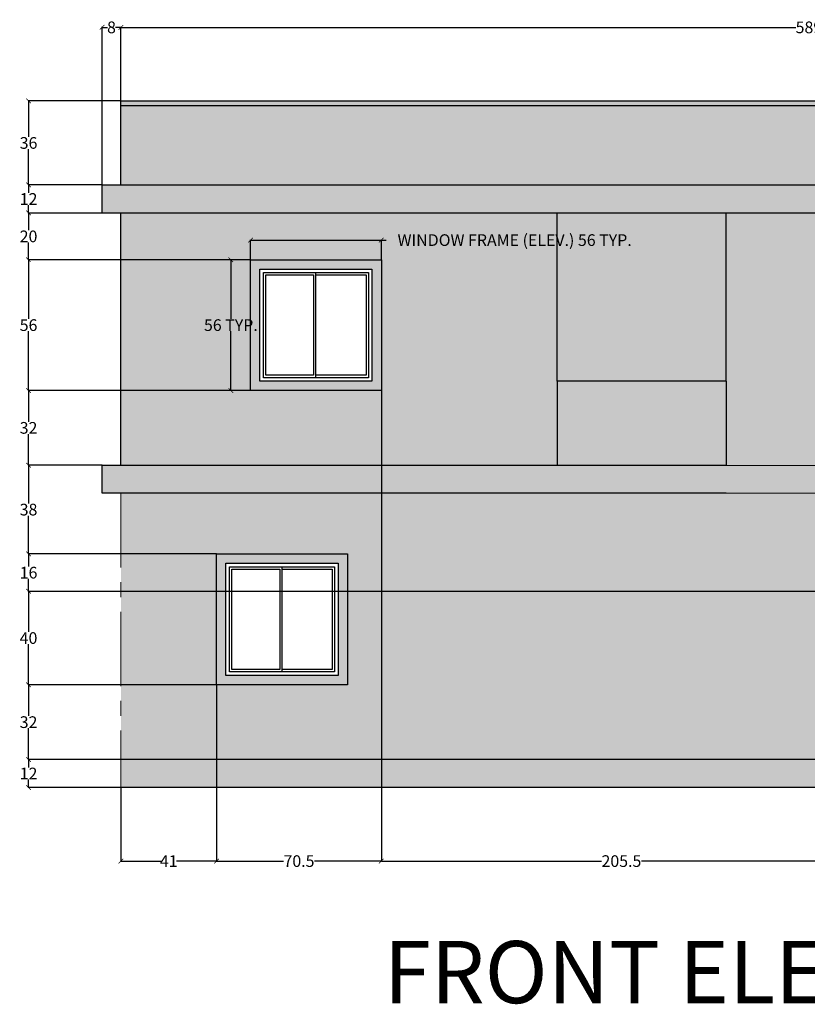
# Model space of a CAD drawing. Units: inches. Extents: x 1455 to 5994, y -182 to 2370.
# Tile 5 of 8: x 4241 to 4579, y -182 to 240. Entities that reach past the tile are written whole.
import ezdxf

# ---------------------------------------------------------------- set-up
doc = ezdxf.new("R2010")
doc.units = ezdxf.units.IN
doc.header["$MEASUREMENT"] = 0
doc.linetypes.add('CENTER', pattern=[50.8, 31.75, -6.35, 6.35, -6.35])
for name, color, linetype, lineweight in [('A-ANNO-DIMS', 2, 'Continuous', 18), ('A-ANNO-TEXT', 7, 'Continuous', 25), ('A-ELEV', 7, 'Continuous', 25), ('A-ELEV-PATT', 8, 'Continuous', 13), ('A-GRID', 8, 'CENTER', 18)]:
    doc.layers.add(name, color=color, linetype=linetype, lineweight=lineweight)
doc.styles.get("Standard").update_dxf_attribs({"font": 'arial.ttf'})
doc.dimstyles.get("Standard").update_dxf_attribs({"dimtxt": 5, "dimasz": 2, "dimexe": 0.18, "dimexo": 0.0625, "dimgap": 0.09, "dimtad": 0, "dimtih": 1, "dimtoh": 1, "dimdec": 1, "dimzin": 0, "dimdsep": 46, "dimlunit": 3, "dimtxsty": 'Standard', "dimblk": 'ARCHTICK', "dimcen": 0.09, "dimadec": 0, "dimazin": 0, "dimtfac": 1, "dimtdec": 1, "dimtofl": 0, "dimtmove": 0, "dimatfit": 3, "dimfxl": 1, "dimtolj": 1, "dimtzin": 0, "dimarcsym": 0})

# ---------------------------------------------------------------- blocks, each defined once
blk = doc.blocks.new('*U8')
for p, q in [((1.5, 1.5), (1.5, 46.5)), ((1.5, 46.5), (24, 46.5)), ((24, 1.5), (24, 46.5)), ((24, 46.5), (46.5, 46.5)), ((46.5, 46.5), (46.5, 1.5)), ((24, 1.5), (1.5, 1.5)), ((46.5, 1.5), (24, 1.5))]:
    blk.add_line(p, q)
blk.add_lwpolyline([(0, 0), (0, 48), (48, 48), (48, 0)], close=True)
for points in [[(23, 45.5), (23, 2.5), (2.5, 2.5), (2.5, 45.5), (23, 45.5)], [(24, 45.5), (45.5, 45.5), (45.5, 2.5), (24, 2.5)]]:
    blk.add_lwpolyline(points)
blk = doc.blocks.new('WIN-FRAME-ELEV')
for p, q in [((0, 0), (0, 56)), ((0, 56), (4, 56)), ((4, 56), (52, 56)), ((52, 56), (56, 56)), ((56, 56), (56, 4)), ((56, 4), (56, 0)), ((4, 0), (0, 0)), ((56, 0), (4, 0))]:
    blk.add_line(p, q)
blk = doc.blocks.new('_ArchTick')
at = {"color": 0, "linetype": 'ByBlock', "const_width": 0.15}
blk.add_lwpolyline([(-0.5, -0.5), (0.5, 0.5)], dxfattribs=at)
blk = doc.blocks.new('*D31')
at = {"layer": 'A-ANNO-DIMS', "color": 0, "lineweight": -2, "transparency": 16777216}
for p, q in [((4340.19, 137.16), (4340.19, 145.68)), ((4340.19, 145.5), (4396.19, 145.5)), ((4396.19, 137.16), (4396.19, 145.68)), ((4396.19, 145.5), (4398.19, 145.5))]:
    blk.add_line(p, q, dxfattribs=at)
at = {"layer": 'Defpoints', "color": 0, "lineweight": 25, "transparency": 16777216}
for p in [(4396.19, 145.5), (4340.19, 137.1), (4396.19, 137.1)]:
    blk.add_point(p, dxfattribs=at)
at = {"layer": 'A-ANNO-DIMS', "color": 0, "lineweight": -2, "transparency": 16777216, "xscale": 2, "yscale": 2, "zscale": 2, "rotation": 180}
blk.add_blockref('_ArchTick', (4340.19, 145.5), dxfattribs=at)
at = {"layer": 'A-ANNO-DIMS', "color": 0, "lineweight": -2, "transparency": 16777216, "xscale": 2, "yscale": 2, "zscale": 2}
blk.add_blockref('_ArchTick', (4396.19, 145.5), dxfattribs=at)
at = {"layer": 'A-ANNO-DIMS', "color": 0, "transparency": 16777216, "insert": (4453.24, 145.5), "char_height": 5, "attachment_point": 5}
blk.add_mtext('\\A1;WINDOW FRAME (ELEV.) 56 TYP.', dxfattribs=at)
blk = doc.blocks.new('*D32')
at = {"layer": 'A-ANNO-DIMS', "color": 0, "lineweight": -2, "transparency": 16777216}
for p, q in [((4340.13, 137.1), (4331.61, 137.1)), ((4331.79, 137.1), (4331.79, 111.74)), ((4331.79, 81.1), (4331.79, 106.45)), ((4340.13, 81.1), (4331.61, 81.1))]:
    blk.add_line(p, q, dxfattribs=at)
at = {"layer": 'Defpoints', "color": 0, "lineweight": 25, "transparency": 16777216}
for p in [(4331.79, 137.1), (4340.19, 137.1), (4340.19, 81.1)]:
    blk.add_point(p, dxfattribs=at)
at = {"layer": 'A-ANNO-DIMS', "color": 0, "lineweight": -2, "transparency": 16777216, "xscale": 2, "yscale": 2, "zscale": 2}
for p, rotation in [((4331.79, 137.1), 90), ((4331.79, 81.1), 270)]:
    blk.add_blockref('_ArchTick', p, dxfattribs=dict(at, rotation=rotation))
at = {"layer": 'A-ANNO-DIMS', "color": 0, "transparency": 16777216, "insert": (4331.79, 109.1), "char_height": 5, "attachment_point": 5}
blk.add_mtext('\\A1;56 TYP.', dxfattribs=at)
blk = doc.blocks.new('*D85')
at = {"layer": 'A-ANNO-DIMS', "color": 0, "lineweight": -2, "transparency": 16777216}
for p, q in [((4276.69, 169.16), (4276.69, 236.78)), ((4276.69, 236.6), (4278.95, 236.6)), ((4284.69, 236.6), (4282.43, 236.6)), ((4284.69, 205.16), (4284.69, 236.78))]:
    blk.add_line(p, q, dxfattribs=at)
at = {"layer": 'Defpoints', "color": 0, "lineweight": 25, "transparency": 16777216}
for p in [(4284.69, 236.6), (4284.69, 205.1), (4276.69, 169.1)]:
    blk.add_point(p, dxfattribs=at)
at = {"layer": 'A-ANNO-DIMS', "color": 0, "lineweight": -2, "transparency": 16777216, "xscale": 2, "yscale": 2, "zscale": 2, "rotation": 180}
blk.add_blockref('_ArchTick', (4276.69, 236.6), dxfattribs=at)
at = {"layer": 'A-ANNO-DIMS', "color": 0, "lineweight": -2, "transparency": 16777216, "xscale": 2, "yscale": 2, "zscale": 2}
blk.add_blockref('_ArchTick', (4284.69, 236.6), dxfattribs=at)
at = {"layer": 'A-ANNO-DIMS', "color": 0, "transparency": 16777216, "insert": (4280.69, 236.6), "char_height": 5, "attachment_point": 5}
blk.add_mtext('\\A1;8', dxfattribs=at)
blk = doc.blocks.new('*D86')
at = {"layer": 'A-ANNO-DIMS', "color": 0, "lineweight": -2, "transparency": 16777216}
for p, q in [((4284.69, 205.16), (4284.69, 236.78)), ((4284.69, 236.6), (4573.57, 236.6)), ((4873.69, 236.6), (4584.81, 236.6)), ((4873.69, 205.16), (4873.69, 236.78))]:
    blk.add_line(p, q, dxfattribs=at)
at = {"layer": 'Defpoints', "color": 0, "lineweight": 25, "transparency": 16777216}
for p in [(4873.69, 236.6), (4284.69, 205.1), (4873.69, 205.1)]:
    blk.add_point(p, dxfattribs=at)
at = {"layer": 'A-ANNO-DIMS', "color": 0, "lineweight": -2, "transparency": 16777216, "xscale": 2, "yscale": 2, "zscale": 2, "rotation": 180}
blk.add_blockref('_ArchTick', (4284.69, 236.6), dxfattribs=at)
at = {"layer": 'A-ANNO-DIMS', "color": 0, "lineweight": -2, "transparency": 16777216, "xscale": 2, "yscale": 2, "zscale": 2}
blk.add_blockref('_ArchTick', (4873.69, 236.6), dxfattribs=at)
at = {"layer": 'A-ANNO-DIMS', "color": 0, "transparency": 16777216, "insert": (4579.19, 236.6), "char_height": 5, "attachment_point": 5}
blk.add_mtext('\\A1;589', dxfattribs=at)
blk = doc.blocks.new('*D87')
at = {"layer": 'A-ANNO-DIMS', "color": 0, "lineweight": -2, "transparency": 16777216}
for p, q in [((4325.69, -44.97), (4325.69, -120.58)), ((4284.69, -88.97), (4284.69, -120.58)), ((4284.69, -120.4), (4301.9, -120.4)), ((4325.69, -120.4), (4308.48, -120.4))]:
    blk.add_line(p, q, dxfattribs=at)
at = {"layer": 'Defpoints', "color": 0, "lineweight": 25, "transparency": 16777216}
for p in [(4325.69, -44.9), (4284.69, -88.9), (4325.69, -120.4)]:
    blk.add_point(p, dxfattribs=at)
at = {"layer": 'A-ANNO-DIMS', "color": 0, "lineweight": -2, "transparency": 16777216, "xscale": 2, "yscale": 2, "zscale": 2, "rotation": 180}
blk.add_blockref('_ArchTick', (4284.69, -120.4), dxfattribs=at)
at = {"layer": 'A-ANNO-DIMS', "color": 0, "lineweight": -2, "transparency": 16777216, "xscale": 2, "yscale": 2, "zscale": 2}
blk.add_blockref('_ArchTick', (4325.69, -120.4), dxfattribs=at)
at = {"layer": 'A-ANNO-DIMS', "color": 0, "transparency": 16777216, "insert": (4305.19, -120.4), "char_height": 5, "attachment_point": 5}
blk.add_mtext('\\A1;41', dxfattribs=at)
blk = doc.blocks.new('*D88')
at = {"layer": 'A-ANNO-DIMS', "color": 0, "lineweight": -2, "transparency": 16777216}
for p, q in [((4396.19, 81.03), (4396.19, -120.58)), ((4325.69, -44.97), (4325.69, -120.58)), ((4325.69, -120.4), (4354.36, -120.4)), ((4396.19, -120.4), (4367.52, -120.4))]:
    blk.add_line(p, q, dxfattribs=at)
at = {"layer": 'Defpoints', "color": 0, "lineweight": 25, "transparency": 16777216}
for p in [(4396.19, 81.1), (4325.69, -44.9), (4396.19, -120.4)]:
    blk.add_point(p, dxfattribs=at)
at = {"layer": 'A-ANNO-DIMS', "color": 0, "lineweight": -2, "transparency": 16777216, "xscale": 2, "yscale": 2, "zscale": 2, "rotation": 180}
blk.add_blockref('_ArchTick', (4325.69, -120.4), dxfattribs=at)
at = {"layer": 'A-ANNO-DIMS', "color": 0, "lineweight": -2, "transparency": 16777216, "xscale": 2, "yscale": 2, "zscale": 2}
blk.add_blockref('_ArchTick', (4396.19, -120.4), dxfattribs=at)
at = {"layer": 'A-ANNO-DIMS', "color": 0, "transparency": 16777216, "insert": (4360.94, -120.4), "char_height": 5, "attachment_point": 5}
blk.add_mtext('\\A1;70.5', dxfattribs=at)
blk = doc.blocks.new('*D89')
at = {"layer": 'A-ANNO-DIMS', "color": 0, "lineweight": -2, "transparency": 16777216}
for p, q in [((4396.19, 81.03), (4396.19, -120.58)), ((4601.69, 81.03), (4601.69, -120.58)), ((4396.19, -120.4), (4490.35, -120.4)), ((4601.69, -120.4), (4507.53, -120.4))]:
    blk.add_line(p, q, dxfattribs=at)
at = {"layer": 'Defpoints', "color": 0, "lineweight": 25, "transparency": 16777216}
for p in [(4396.19, 81.1), (4601.69, 81.1), (4601.69, -120.4)]:
    blk.add_point(p, dxfattribs=at)
at = {"layer": 'A-ANNO-DIMS', "color": 0, "lineweight": -2, "transparency": 16777216, "xscale": 2, "yscale": 2, "zscale": 2, "rotation": 180}
blk.add_blockref('_ArchTick', (4396.19, -120.4), dxfattribs=at)
at = {"layer": 'A-ANNO-DIMS', "color": 0, "lineweight": -2, "transparency": 16777216, "xscale": 2, "yscale": 2, "zscale": 2}
blk.add_blockref('_ArchTick', (4601.69, -120.4), dxfattribs=at)
at = {"layer": 'A-ANNO-DIMS', "color": 0, "transparency": 16777216, "insert": (4498.94, -120.4), "char_height": 5, "attachment_point": 5}
blk.add_mtext('\\A1;205.5', dxfattribs=at)
blk = doc.blocks.new('*D96')
at = {"layer": 'A-ANNO-DIMS', "color": 0, "lineweight": -2, "transparency": 16777216}
for p, q in [((4284.63, -76.9), (4245.01, -76.9)), ((4245.19, -76.9), (4245.19, -80.3)), ((4245.19, -88.9), (4245.19, -85.5)), ((4284.63, -88.9), (4245.01, -88.9))]:
    blk.add_line(p, q, dxfattribs=at)
at = {"layer": 'Defpoints', "color": 0, "lineweight": 25, "transparency": 16777216}
for p in [(4245.19, -76.9), (4284.69, -76.9), (4284.69, -88.9)]:
    blk.add_point(p, dxfattribs=at)
at = {"layer": 'A-ANNO-DIMS', "color": 0, "lineweight": -2, "transparency": 16777216, "xscale": 2, "yscale": 2, "zscale": 2}
for p, rotation in [((4245.19, -76.9), 90), ((4245.19, -88.9), 270)]:
    blk.add_blockref('_ArchTick', p, dxfattribs=dict(at, rotation=rotation))
at = {"layer": 'A-ANNO-DIMS', "color": 0, "transparency": 16777216, "insert": (4245.19, -82.9), "char_height": 5, "attachment_point": 5}
blk.add_mtext('\\A1;12', dxfattribs=at)
blk = doc.blocks.new('*D97')
at = {"layer": 'A-ANNO-DIMS', "color": 0, "lineweight": -2, "transparency": 16777216}
for p, q in [((4325.63, -44.9), (4245.01, -44.9)), ((4245.19, -44.9), (4245.19, -58.26)), ((4245.19, -76.9), (4245.19, -63.55)), ((4284.63, -76.9), (4245.01, -76.9))]:
    blk.add_line(p, q, dxfattribs=at)
at = {"layer": 'Defpoints', "color": 0, "lineweight": 25, "transparency": 16777216}
for p in [(4245.19, -44.9), (4325.69, -44.9), (4284.69, -76.9)]:
    blk.add_point(p, dxfattribs=at)
at = {"layer": 'A-ANNO-DIMS', "color": 0, "lineweight": -2, "transparency": 16777216, "xscale": 2, "yscale": 2, "zscale": 2}
for p, rotation in [((4245.19, -44.9), 90), ((4245.19, -76.9), 270)]:
    blk.add_blockref('_ArchTick', p, dxfattribs=dict(at, rotation=rotation))
at = {"layer": 'A-ANNO-DIMS', "color": 0, "transparency": 16777216, "insert": (4245.19, -60.9), "char_height": 5, "attachment_point": 5}
blk.add_mtext('\\A1;32', dxfattribs=at)
blk = doc.blocks.new('*D98')
at = {"layer": 'A-ANNO-DIMS', "color": 0, "lineweight": -2, "transparency": 16777216}
for p, q in [((4619.63, -4.9), (4245.01, -4.9)), ((4245.19, -4.9), (4245.19, -22.26)), ((4245.19, -44.9), (4245.19, -27.55)), ((4325.63, -44.9), (4245.01, -44.9))]:
    blk.add_line(p, q, dxfattribs=at)
at = {"layer": 'Defpoints', "color": 0, "lineweight": 25, "transparency": 16777216}
for p in [(4245.19, -4.9), (4619.69, -4.9), (4325.69, -44.9)]:
    blk.add_point(p, dxfattribs=at)
at = {"layer": 'A-ANNO-DIMS', "color": 0, "lineweight": -2, "transparency": 16777216, "xscale": 2, "yscale": 2, "zscale": 2}
for p, rotation in [((4245.19, -4.9), 90), ((4245.19, -44.9), 270)]:
    blk.add_blockref('_ArchTick', p, dxfattribs=dict(at, rotation=rotation))
at = {"layer": 'A-ANNO-DIMS', "color": 0, "transparency": 16777216, "insert": (4245.19, -24.9), "char_height": 5, "attachment_point": 5}
blk.add_mtext('\\A1;40', dxfattribs=at)
blk = doc.blocks.new('*D99')
at = {"layer": 'A-ANNO-DIMS', "color": 0, "lineweight": -2, "transparency": 16777216}
for p, q in [((4325.63, 11.1), (4245.01, 11.1)), ((4245.19, 11.1), (4245.19, 5.74)), ((4245.19, -4.9), (4245.19, 0.45)), ((4619.63, -4.9), (4245.01, -4.9))]:
    blk.add_line(p, q, dxfattribs=at)
at = {"layer": 'Defpoints', "color": 0, "lineweight": 25, "transparency": 16777216}
for p in [(4245.19, 11.1), (4325.69, 11.1), (4619.69, -4.9)]:
    blk.add_point(p, dxfattribs=at)
at = {"layer": 'A-ANNO-DIMS', "color": 0, "lineweight": -2, "transparency": 16777216, "xscale": 2, "yscale": 2, "zscale": 2}
for p, rotation in [((4245.19, 11.1), 90), ((4245.19, -4.9), 270)]:
    blk.add_blockref('_ArchTick', p, dxfattribs=dict(at, rotation=rotation))
at = {"layer": 'A-ANNO-DIMS', "color": 0, "transparency": 16777216, "insert": (4245.19, 3.1), "char_height": 5, "attachment_point": 5}
blk.add_mtext('\\A1;16', dxfattribs=at)
blk = doc.blocks.new('*D100')
at = {"layer": 'A-ANNO-DIMS', "color": 0, "lineweight": -2, "transparency": 16777216}
for p, q in [((4276.63, 49.1), (4245.01, 49.1)), ((4245.19, 49.1), (4245.19, 32.74)), ((4245.19, 11.1), (4245.19, 27.45)), ((4325.63, 11.1), (4245.01, 11.1))]:
    blk.add_line(p, q, dxfattribs=at)
at = {"layer": 'Defpoints', "color": 0, "lineweight": 25, "transparency": 16777216}
for p in [(4245.19, 49.1), (4276.69, 49.1), (4325.69, 11.1)]:
    blk.add_point(p, dxfattribs=at)
at = {"layer": 'A-ANNO-DIMS', "color": 0, "lineweight": -2, "transparency": 16777216, "xscale": 2, "yscale": 2, "zscale": 2}
for p, rotation in [((4245.19, 49.1), 90), ((4245.19, 11.1), 270)]:
    blk.add_blockref('_ArchTick', p, dxfattribs=dict(at, rotation=rotation))
at = {"layer": 'A-ANNO-DIMS', "color": 0, "transparency": 16777216, "insert": (4245.19, 30.1), "char_height": 5, "attachment_point": 5}
blk.add_mtext('\\A1;38', dxfattribs=at)
blk = doc.blocks.new('*D101')
at = {"layer": 'A-ANNO-DIMS', "color": 0, "lineweight": -2, "transparency": 16777216}
for p, q in [((4340.13, 81.1), (4245.01, 81.1)), ((4245.19, 81.1), (4245.19, 67.74)), ((4245.19, 49.1), (4245.19, 62.45)), ((4276.63, 49.1), (4245.01, 49.1))]:
    blk.add_line(p, q, dxfattribs=at)
at = {"layer": 'Defpoints', "color": 0, "lineweight": 25, "transparency": 16777216}
for p in [(4245.19, 81.1), (4340.19, 81.1), (4276.69, 49.1)]:
    blk.add_point(p, dxfattribs=at)
at = {"layer": 'A-ANNO-DIMS', "color": 0, "lineweight": -2, "transparency": 16777216, "xscale": 2, "yscale": 2, "zscale": 2}
for p, rotation in [((4245.19, 81.1), 90), ((4245.19, 49.1), 270)]:
    blk.add_blockref('_ArchTick', p, dxfattribs=dict(at, rotation=rotation))
at = {"layer": 'A-ANNO-DIMS', "color": 0, "transparency": 16777216, "insert": (4245.19, 65.1), "char_height": 5, "attachment_point": 5}
blk.add_mtext('\\A1;32', dxfattribs=at)
blk = doc.blocks.new('*D102')
at = {"layer": 'A-ANNO-DIMS', "color": 0, "lineweight": -2, "transparency": 16777216}
for p, q in [((4340.13, 137.1), (4245.01, 137.1)), ((4245.19, 137.1), (4245.19, 111.74)), ((4245.19, 81.1), (4245.19, 106.45)), ((4340.13, 81.1), (4245.01, 81.1))]:
    blk.add_line(p, q, dxfattribs=at)
at = {"layer": 'Defpoints', "color": 0, "lineweight": 25, "transparency": 16777216}
for p in [(4245.19, 137.1), (4340.19, 137.1), (4340.19, 81.1)]:
    blk.add_point(p, dxfattribs=at)
at = {"layer": 'A-ANNO-DIMS', "color": 0, "lineweight": -2, "transparency": 16777216, "xscale": 2, "yscale": 2, "zscale": 2}
for p, rotation in [((4245.19, 137.1), 90), ((4245.19, 81.1), 270)]:
    blk.add_blockref('_ArchTick', p, dxfattribs=dict(at, rotation=rotation))
at = {"layer": 'A-ANNO-DIMS', "color": 0, "transparency": 16777216, "insert": (4245.19, 109.1), "char_height": 5, "attachment_point": 5}
blk.add_mtext('\\A1;56', dxfattribs=at)
blk = doc.blocks.new('*D103')
at = {"layer": 'A-ANNO-DIMS', "color": 0, "lineweight": -2, "transparency": 16777216}
for p, q in [((4276.63, 157.1), (4245.01, 157.1)), ((4245.19, 157.1), (4245.19, 149.74)), ((4245.19, 137.1), (4245.19, 144.45)), ((4340.13, 137.1), (4245.01, 137.1))]:
    blk.add_line(p, q, dxfattribs=at)
at = {"layer": 'Defpoints', "color": 0, "lineweight": 25, "transparency": 16777216}
for p in [(4245.19, 157.1), (4276.69, 157.1), (4340.19, 137.1)]:
    blk.add_point(p, dxfattribs=at)
at = {"layer": 'A-ANNO-DIMS', "color": 0, "lineweight": -2, "transparency": 16777216, "xscale": 2, "yscale": 2, "zscale": 2}
for p, rotation in [((4245.19, 157.1), 90), ((4245.19, 137.1), 270)]:
    blk.add_blockref('_ArchTick', p, dxfattribs=dict(at, rotation=rotation))
at = {"layer": 'A-ANNO-DIMS', "color": 0, "transparency": 16777216, "insert": (4245.19, 147.1), "char_height": 5, "attachment_point": 5}
blk.add_mtext('\\A1;20', dxfattribs=at)
blk = doc.blocks.new('*D104')
at = {"layer": 'A-ANNO-DIMS', "color": 0, "lineweight": -2, "transparency": 16777216}
for p, q in [((4276.63, 169.1), (4245.01, 169.1)), ((4245.19, 169.1), (4245.19, 165.7)), ((4245.19, 157.1), (4245.19, 160.5)), ((4276.63, 157.1), (4245.01, 157.1))]:
    blk.add_line(p, q, dxfattribs=at)
at = {"layer": 'Defpoints', "color": 0, "lineweight": 25, "transparency": 16777216}
for p in [(4245.19, 169.1), (4276.69, 169.1), (4276.69, 157.1)]:
    blk.add_point(p, dxfattribs=at)
at = {"layer": 'A-ANNO-DIMS', "color": 0, "lineweight": -2, "transparency": 16777216, "xscale": 2, "yscale": 2, "zscale": 2}
for p, rotation in [((4245.19, 169.1), 90), ((4245.19, 157.1), 270)]:
    blk.add_blockref('_ArchTick', p, dxfattribs=dict(at, rotation=rotation))
at = {"layer": 'A-ANNO-DIMS', "color": 0, "transparency": 16777216, "insert": (4245.19, 163.1), "char_height": 5, "attachment_point": 5}
blk.add_mtext('\\A1;12', dxfattribs=at)
blk = doc.blocks.new('*D105')
at = {"layer": 'A-ANNO-DIMS', "color": 0, "lineweight": -2, "transparency": 16777216}
for p, q in [((4284.63, 205.1), (4245.01, 205.1)), ((4245.19, 205.1), (4245.19, 189.74)), ((4245.19, 169.1), (4245.19, 184.45)), ((4276.63, 169.1), (4245.01, 169.1))]:
    blk.add_line(p, q, dxfattribs=at)
at = {"layer": 'Defpoints', "color": 0, "lineweight": 25, "transparency": 16777216}
for p in [(4245.19, 205.1), (4284.69, 205.1), (4276.69, 169.1)]:
    blk.add_point(p, dxfattribs=at)
at = {"layer": 'A-ANNO-DIMS', "color": 0, "lineweight": -2, "transparency": 16777216, "xscale": 2, "yscale": 2, "zscale": 2}
for p, rotation in [((4245.19, 205.1), 90), ((4245.19, 169.1), 270)]:
    blk.add_blockref('_ArchTick', p, dxfattribs=dict(at, rotation=rotation))
at = {"layer": 'A-ANNO-DIMS', "color": 0, "transparency": 16777216, "insert": (4245.19, 187.1), "char_height": 5, "attachment_point": 5}
blk.add_mtext('\\A1;36', dxfattribs=at)

msp = doc.modelspace()

# ---------------------------------------------------------------- hatches: boundary and pattern name
at = {"layer": 'A-ELEV-PATT', "transparency": 33554641}
h = msp.add_hatch(color=256, dxfattribs=at)
h.dxf.hatch_style = 1
h.paths.add_polyline_path([(4873.6884, 205.0969), (4284.6884, 205.0969), (4284.6884, 203.0969), (4873.6884, 203.0969)])
h = msp.add_hatch(color=256, dxfattribs=at)
h.dxf.hatch_style = 1
h.paths.add_polyline_path([(4873.6884, 203.0969), (4284.6884, 203.0969), (4284.6884, 169.0969), (4768.6884, 169.0969), (4864.6884, 169.0969), (4873.6884, 169.0969)])
h = msp.add_hatch(color=256, dxfattribs=at)
h.dxf.hatch_style = 1
h.paths.add_polyline_path([(4768.6884, 169.0969), (4284.6884, 169.0969), (4276.6884, 169.0969), (4276.6884, 157.0969), (4756.6884, 157.0969), (4756.6884, 49.0187), (4719.7422, 49.0288), (4719.7422, 49.0261), (4713.167, 49.0261), (4704.4367, 49.0287), (4704.4367, 49.0261), (4697.8615, 49.0261), (4689.1312, 49.0288), (4689.1312, 49.0261), (4682.556, 49.0261), (4673.8258, 49.029), (4673.8258, 49.0261), (4667.2505, 49.0261), (4471.4513, 49.0969), (4284.6884, 49.0969), (4276.6884, 49.0969), (4276.6884, 37.0915), (4543.7991, 37.0915), (4768.6843, 37.0146)])
h = msp.add_hatch(color=256, dxfattribs=at)
h.dxf.hatch_style = 1
h.paths.add_polyline_path([(4873.6884, 169.0969), (4864.6884, 169.0969), (4864.6884, 85.0969), (4864.6884, 49.0146), (4864.6884, 43.0969), (4864.6884, -70.9031), (4864.6884, -76.9031), (4861.6884, -76.9031), (4837.6884, -76.9031), (4834.6884, -76.9031), (4768.6884, -76.9031), (4763.6884, -76.9031), (4284.6884, -76.9031), (4284.6884, -88.9031), (4873.6884, -88.9031)])
h = msp.add_hatch(color=256, dxfattribs=at)
h.dxf.hatch_style = 1
h.paths.add_polyline_path([(4471.4513, 157.0969), (4284.6884, 157.0969), (4284.6884, 49.0969), (4471.4513, 49.0969), (4471.4513, 85.0969)])
h.paths.add_polyline_path([(4396.1884, 85.0969), (4396.1884, 81.0969), (4344.1884, 81.0969), (4340.1884, 81.0969), (4340.1884, 137.0969), (4344.1884, 137.0969), (4392.1884, 137.0969), (4396.1884, 137.0969)], flags=16)
h.paths.add_polyline_path([(4607.6884, 37.0697), (4543.7991, 37.0915), (4284.6884, 37.0915), (4284.6884, -76.9031), (4607.6884, -76.9031)])
h.paths.add_polyline_path([(4381.6884, -40.9031), (4381.6884, -44.9031), (4329.6884, -44.9031), (4325.6884, -44.9031), (4325.6884, 11.0969), (4329.6884, 11.0969), (4377.6884, 11.0969), (4381.6884, 11.0969)], flags=16)
h.paths.add_polyline_path([(4377.6884, -40.9031), (4329.6884, -40.9031), (4329.6884, 7.0969), (4377.6884, 7.0969)], flags=0)
h.paths.add_polyline_path([(4376.1884, -39.4031), (4353.6884, -39.4031), (4331.1884, -39.4031), (4331.1884, 5.5969), (4353.6884, 5.5969), (4376.1884, 5.5969)], flags=0)
h.paths.add_polyline_path([(4375.1884, -38.4031), (4353.6884, -38.4031), (4353.6884, 4.5969), (4375.1884, 4.5969)], flags=0)
h.paths.add_polyline_path([(4352.6884, -38.4031), (4332.1884, -38.4031), (4332.1884, 4.5969), (4352.6884, 4.5969)], flags=0)
h.paths.add_polyline_path([(4667.2505, 157.0969), (4543.8032, 157.0969), (4543.8032, 85.0969), (4543.8032, 49.0771), (4667.2505, 49.0432)])
h.paths.add_polyline_path([(4601.6884, 81.0969), (4601.6884, 137.0969), (4605.6884, 137.0969), (4653.6884, 137.0969), (4657.6884, 137.0969), (4657.6884, 81.0969)], flags=16)
h.paths.add_polyline_path([(4543.8032, 157.0969), (4471.4513, 157.0969), (4471.4513, 85.0969), (4543.8032, 85.0969)])
h.paths.add_polyline_path([(4763.6884, 37.0163), (4619.6884, 37.0656), (4619.6884, -4.9031), (4643.6884, -4.9031), (4667.6884, -4.9031), (4667.6884, -76.9031), (4763.6884, -76.9031)])
h.paths.add_polyline_path([(4864.6884, 43.0969), (4768.6884, 43.0969), (4768.6884, -76.9031), (4834.6884, -76.9031), (4834.6884, -4.9031), (4864.6884, -4.9031)])
h = msp.add_hatch(color=256, dxfattribs=at)
h.dxf.hatch_style = 1
h.paths.add_polyline_path([(4396.1884, 137.0969), (4392.1884, 137.0969), (4344.1884, 137.0969), (4340.1884, 137.0969), (4340.1884, 81.0969), (4344.1884, 81.0969), (4396.1884, 81.0969), (4396.1884, 85.0969)])
h.paths.add_polyline_path([(4344.1884, 133.0969), (4392.1884, 133.0969), (4392.1884, 85.0969), (4344.1884, 85.0969)], flags=16)
h.paths.add_polyline_path([(4345.6884, 131.5969), (4368.1884, 131.5969), (4390.6884, 131.5969), (4390.6884, 86.5969), (4368.1884, 86.5969), (4345.6884, 86.5969)], flags=0)
h.paths.add_polyline_path([(4346.6884, 130.5969), (4367.1884, 130.5969), (4367.1884, 87.5969), (4346.6884, 87.5969)], flags=0)
h.paths.add_polyline_path([(4368.1884, 130.5969), (4389.6884, 130.5969), (4389.6884, 87.5969), (4368.1884, 87.5969)], flags=0)
h.paths.add_polyline_path([(4657.6884, 137.0969), (4653.6884, 137.0969), (4605.6884, 137.0969), (4601.6884, 137.0969), (4601.6884, 81.0969), (4657.6884, 81.0969)])
h.paths.add_polyline_path([(4653.6884, 133.0969), (4653.6884, 85.0969), (4605.6884, 85.0969), (4605.6884, 133.0969)], flags=16)
h.paths.add_polyline_path([(4629.6884, 131.5969), (4652.1884, 131.5969), (4652.1884, 86.5969), (4629.6884, 86.5969), (4607.1884, 86.5969), (4607.1884, 131.5969)], flags=0)
h.paths.add_polyline_path([(4628.6884, 130.5969), (4628.6884, 87.5969), (4608.1884, 87.5969), (4608.1884, 130.5969)], flags=0)
h.paths.add_polyline_path([(4629.6884, 130.5969), (4651.1884, 130.5969), (4651.1884, 87.5969), (4629.6884, 87.5969)], flags=0)
h.paths.add_polyline_path([(4381.6884, 11.0969), (4377.6884, 11.0969), (4329.6884, 11.0969), (4325.6884, 11.0969), (4325.6884, -44.9031), (4329.6884, -44.9031), (4381.6884, -44.9031), (4381.6884, -40.9031)])
h.paths.add_polyline_path([(4377.6884, 7.0969), (4377.6884, -40.9031), (4329.6884, -40.9031), (4329.6884, 7.0969)], flags=16)
h.paths.add_polyline_path([(4353.6884, 5.5969), (4376.1884, 5.5969), (4376.1884, -39.4031), (4353.6884, -39.4031), (4331.1884, -39.4031), (4331.1884, 5.5969)], flags=0)
h.paths.add_polyline_path([(4353.6884, 4.5969), (4375.1884, 4.5969), (4375.1884, -38.4031), (4353.6884, -38.4031)], flags=0)
h.paths.add_polyline_path([(4352.6884, -38.4031), (4332.1884, -38.4031), (4332.1884, 4.5969), (4352.6884, 4.5969)], flags=0)
at = {"layer": 'A-ELEV-PATT', "transparency": 33554666}
h = msp.add_hatch(color=256, dxfattribs=at)
h.dxf.hatch_style = 1
h.paths.add_polyline_path([(4864.6884, 85.0969), (4768.6884, 85.0969), (4768.6884, 49.0969), (4864.6884, 49.0969)])
h.paths.add_polyline_path([(4543.8032, 85.0969), (4471.4513, 85.0969), (4471.4513, 49.0969), (4543.8032, 49.0969)])

# ---------------------------------------------------------------- linework, layer by layer
at = {"layer": 'A-ELEV'}
for p, q in [((4284.6884, 169.0969), (4284.6884, 205.0969)), ((4284.6884, 205.0969), (4873.6884, 205.0969)), ((4284.6884, 203.0969), (4873.6884, 203.0969)), ((4284.6884, 49.0969), (4284.6884, 157.0969)), ((4471.4513, 85.0969), (4471.4513, 157.0969)), ((4543.8032, 85.0969), (4543.8032, 157.0969)), ((4471.4513, 85.0969), (4471.4513, 49.0969)), ((4543.8032, 85.0969), (4471.4513, 85.0969)), ((4543.8032, 85.0969), (4543.8032, 49.0915)), ((4471.4513, 49.0969), (4543.8032, 49.0969)), ((4763.6884, -76.9031), (4284.6884, -76.9031)), ((4873.6884, -88.9031), (4284.6884, -88.9031))]:
    msp.add_line(p, q, dxfattribs=at)
msp.add_lwpolyline([(4756.6884, 49.0146), (4756.6884, 157.0969), (4276.6884, 157.0969), (4276.6884, 169.0969), (4284.6884, 169.0969), (4768.6884, 169.0969), (4768.6843, 37.0146), (4543.7991, 37.0915), (4276.6884, 37.0915), (4276.6884, 49.0969), (4284.6884, 49.0969), (4471.4513, 49.0969), (4756.6884, 49.0187)], dxfattribs=at)
at = {"layer": 'A-GRID'}
msp.add_line((4284.6884, 37.0915), (4284.6884, -88.9031), dxfattribs=at)

# ---------------------------------------------------------------- block references
at = {"layer": 'A-ELEV'}
for name, p in [('WIN-FRAME-ELEV', (4340.188, 81.097)), ('*U8', (4344.1884, 85.0969)), ('WIN-FRAME-ELEV', (4325.688, -44.903)), ('*U8', (4329.6884, -40.9031))]:
    msp.add_blockref(name, p, dxfattribs=at)

# ---------------------------------------------------------------- texts
at = {"layer": 'A-ANNO-TEXT'}
msp.add_text('FRONT ELEVATION', height=26.640459, dxfattribs=at).set_placement((4397.2929, -181.252))

# ---------------------------------------------------------------- dimensions: what is measured, and where the dimension line sits
at = {"layer": 'A-ANNO-DIMS'}
for base, p1, p2, override, picture, middle in [((4284.6884, 236.5969), (4276.6884, 169.0969), (4284.6884, 205.0969), {"dimdec": 0, "dimlfac": 1, "dimrnd": 0, "dimzin": 0, "dimdsep": 46, "dimlunit": 2}, '*D85', (4280.6884, 236.5969)), ((4873.6884, 236.5969), (4284.6884, 205.0969), (4873.6884, 205.0969), {"dimdec": 0, "dimlfac": 1, "dimrnd": 0, "dimzin": 0, "dimdsep": 46, "dimlunit": 2}, '*D86', (4579.1884, 236.5969)), ((4396.1884, -120.4031), (4325.6884, -44.9031), (4396.1884, 81.0969), {"dimdec": 1, "dimlfac": 1, "dimrnd": 0, "dimzin": 0, "dimdsep": 46, "dimlunit": 2}, '*D88', (4360.9384, -120.4031)), ((4601.6884, -120.4031), (4396.1884, 81.0969), (4601.6884, 81.0969), {"dimdec": 1, "dimlfac": 1, "dimrnd": 0, "dimzin": 0, "dimdsep": 46, "dimlunit": 2}, '*D89', (4498.9384, -120.4031)), ((4325.6884, -120.4031), (4284.6884, -88.9031), (4325.6884, -44.9031), {"dimdec": 0, "dimlfac": 1, "dimrnd": 0, "dimzin": 0, "dimdsep": 46, "dimlunit": 2}, '*D87', (4305.1884, -120.4031))]:
    dim = msp.add_linear_dim(base=base, p1=p1, p2=p2, dimstyle='Standard', override=override, dxfattribs=at)
    dim.commit()
    dim.dimension.update_dxf_attribs({"geometry": picture, "text_midpoint": middle})
for base, p1, p2, picture, middle in [((4245.1884, 205.0969), (4276.6884, 169.0969), (4284.6884, 205.0969), '*D105', (4245.1884, 187.0969)), ((4245.1884, 169.0969), (4276.6884, 157.0969), (4276.6884, 169.0969), '*D104', (4245.1884, 163.0969)), ((4245.1884, 157.0969), (4340.1884, 137.0969), (4276.6884, 157.0969), '*D103', (4245.1884, 147.0969)), ((4245.1884, 137.0969), (4340.1884, 81.0969), (4340.1884, 137.0969), '*D102', (4245.1884, 109.0969)), ((4245.1884, 81.0969), (4276.6884, 49.0969), (4340.1884, 81.0969), '*D101', (4245.1884, 65.0969)), ((4245.1884, 49.0969), (4325.6884, 11.0969), (4276.6884, 49.0969), '*D100', (4245.1884, 30.0969)), ((4245.1884, 11.0969), (4619.6884, -4.9031), (4325.6884, 11.0969), '*D99', (4245.1884, 3.0969)), ((4245.1884, -4.9031), (4325.6884, -44.9031), (4619.6884, -4.9031), '*D98', (4245.1884, -24.9031)), ((4245.1884, -44.9031), (4284.6884, -76.9031), (4325.6884, -44.9031), '*D97', (4245.1884, -60.9031)), ((4245.1884, -76.9031), (4284.6884, -88.9031), (4284.6884, -76.9031), '*D96', (4245.1884, -82.9031))]:
    dim = msp.add_linear_dim(base=base, p1=p1, p2=p2, angle=90, dimstyle='Standard', override={"dimdec": 0, "dimlfac": 1, "dimrnd": 0, "dimzin": 0, "dimdsep": 46, "dimlunit": 2}, dxfattribs=at)
    dim.commit()
    dim.dimension.update_dxf_attribs({"geometry": picture, "text_midpoint": middle})
dim = msp.add_linear_dim(base=(4396.1884, 145.4969), p1=(4340.1884, 137.0969), p2=(4396.1884, 137.0969), text='WINDOW FRAME (ELEV.) <> TYP.', dimstyle='Standard', override={"dimdec": 0, "dimlfac": 1, "dimrnd": 0, "dimzin": 0, "dimdsep": 46, "dimlunit": 2}, dxfattribs=at)
dim.commit()
dim.dimension.update_dxf_attribs({"geometry": '*D31', "text_midpoint": (4453.2358, 145.4969)})
dim = msp.add_linear_dim(base=(4331.7884, 137.0969), p1=(4340.1884, 81.0969), p2=(4340.1884, 137.0969), angle=90, text='<> TYP.', dimstyle='Standard', override={"dimdec": 0, "dimlfac": 1, "dimrnd": 0, "dimzin": 0, "dimdsep": 46, "dimlunit": 2}, dxfattribs=at)
dim.commit()
dim.dimension.update_dxf_attribs({"geometry": '*D32', "text_midpoint": (4331.7884, 109.0969)})

doc.saveas('drawing.dxf')
